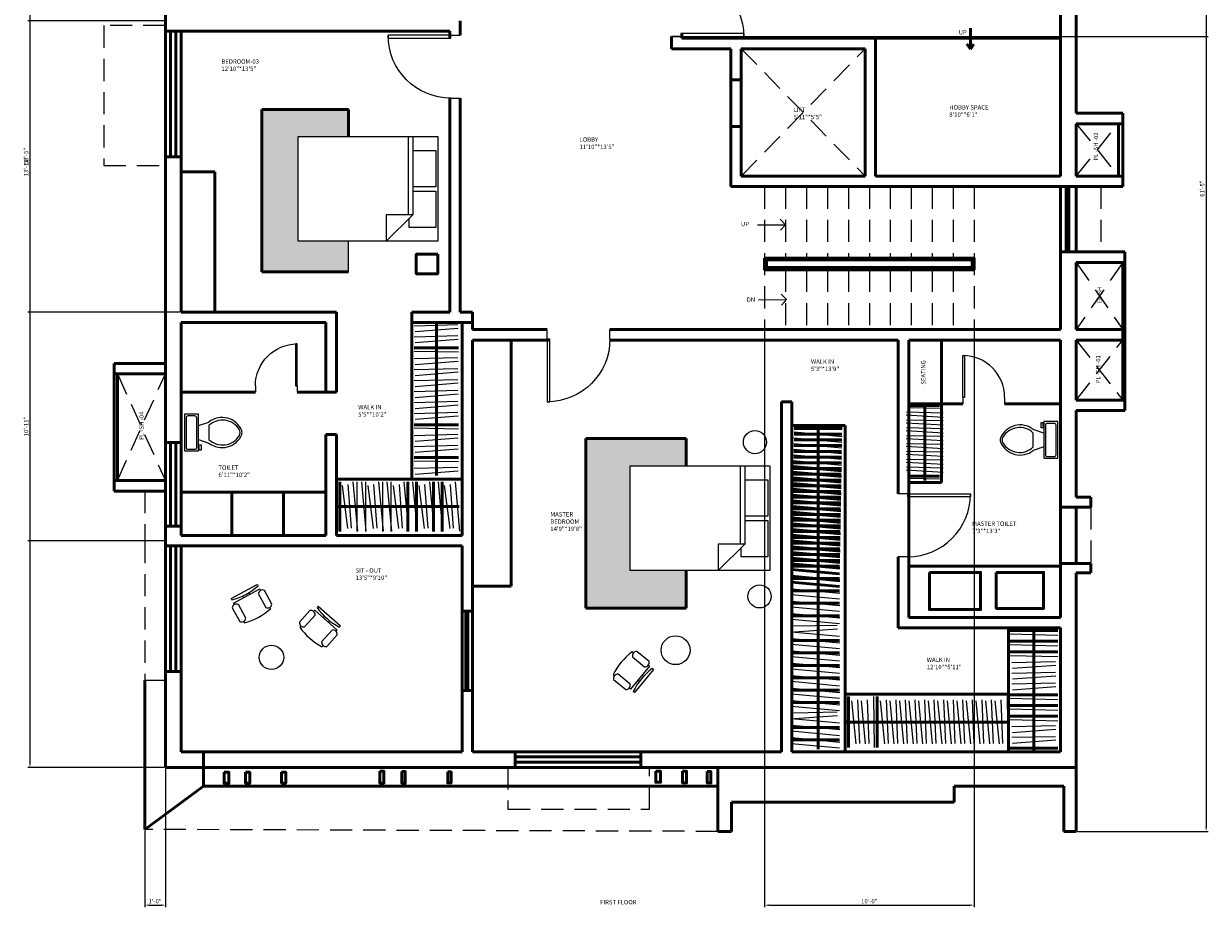
# Model space of a CAD drawing. Units: inches. Extents: x 5312 to 23584, y 2846 to 7447.
# Tile 5 of 12: x 9893 to 10572, y 3045 to 3551. Entities that reach past the tile are written whole.
import ezdxf

# ---------------------------------------------------------------- set-up
doc = ezdxf.new("R2010")
doc.units = ezdxf.units.IN
doc.linetypes.add('DASHED', pattern=[19.05, 12.7, -6.35])
for name, color, linetype, lineweight in [('A-ANNO-DIMS', 2, 'Continuous', 18), ('A-ANNO-TEXT', 3, 'Continuous', 18), ('A-AREA-IDEN', 7, 'Continuous', 18), ('A-DOOR', 4, 'Continuous', 25), ('A-FLOR-FIXT', 9, 'Continuous', 18), ('A-FLOR-OVHD', 8, 'DASHED', 18), ('A-FLOR-PATT', 252, 'Continuous', 13), ('A-FLOR-STRS', 3, 'Continuous', 18), ('A-FURN', 8, 'Continuous', 18), ('A-WALL', 7, 'Continuous', 50)]:
    doc.layers.add(name, color=color, linetype=linetype, lineweight=lineweight)
doc.styles.get("Standard").update_dxf_attribs({"font": 'arial.ttf'})
doc.dimstyles.new('ISO-25', dxfattribs={"dimtxt": 2.5, "dimasz": 2.5, "dimexe": 1.25, "dimexo": 0.625, "dimtad": 1, "dimlunit": 3, "dimtxsty": 'Standard', "dimcen": 2.5, "dimadec": 0, "dimazin": 0, "dimtfac": 1, "dimtmove": 0, "dimatfit": 3, "dimfxl": 1, "dimarcsym": 0})

# ---------------------------------------------------------------- blocks, each defined once
blk = doc.blocks.new('*U2')
for p, q in [((0, 0), (0, -6)), ((40, 0), (40, -6))]:
    blk.add_line(p, q)
blk.add_lwpolyline([(0, 0), (0, 40), (1.75, 40), (1.75, 0)], close=True)
blk.add_arc((0, 0), 40, 0, 90)
blk = doc.blocks.new('Toilet - top')
for p, q in [((9.5, -6), (9.5, -2)), ((-10, -8.5), (-8, -8.5)), ((-10, -9.5), (-10, -8.5)), ((-7, -9.5), (-10, -9.5)), ((-8, -8.5), (-8, -8)), ((-7, -8), (-7, -9.5)), ((-4, -8), (-6, -14)), ((4, -8), (6, -14)), ((4, -14), (-4, -14))]:
    blk.add_line(p, q)
blk.add_lwpolyline([(10.5, -8), (10.5, 0), (-10.5, 0), (-10.5, -8)], close=True)
for points in [[(-9.5, -2), (-9.5, -6)], [(8.5, -1), (-8.5, -1)], [(-8.5, -7), (8.5, -7)]]:
    blk.add_lwpolyline(points)
for centre, radius, start, end in [((-8.62, -1.88), 0.884, 81.8699, 188.1301), ((-8.62, -6.12), 0.884, 171.8699, 278.1301), ((8.62, -1.88), 0.884, 351.8699, 98.1301), ((8.62, -6.12), 0.884, 261.8699, 8.1301), ((3.52, -21.58), 12.17, 141.46911, 247.97143), ((4.2, -21.82), 11.33, 136.36773, 238.94682), ((-3.52, -21.58), 12.17, 292.02843, 38.53071), ((-4.2, -21.82), 11.33, 301.05301, 43.63209), ((0, -27.88), 4, 245.73182, 294.26817), ((0, -29), 4, 254.86053, 285.13947)]:
    blk.add_arc(centre, radius, start, end)
blk = doc.blocks.new('Bed - Queen')
for p, q in [((0, -80.00003), (0, 0)), ((0, 0), (59.99999, 0)), ((59.99999, 0), (59.99999, -80.00003)), ((7.99999, -1.2), (28.79998, -1.2)), ((7.99999, -14.4), (7.99999, -1.2)), ((28.79998, -1.2), (28.79998, -14.4)), ((31.19999, -1.2), (51.99999, -1.2)), ((31.19999, -14.4), (31.19999, -1.2)), ((51.99999, -1.2), (51.99999, -16.4)), ((0, -14.4), (44.8, -14.4)), ((44.8, -16.8), (0, -16.8)), ((59.99999, -29.6), (44.8, -14.4)), ((44.8, -14.4), (44.8, -29.6)), ((51.99999, -16.4), (46.79936, -16.4)), ((44.8, -29.6), (59.99999, -29.6)), ((59.99999, -80.00003), (0, -80.00003))]:
    blk.add_line(p, q)
blk = doc.blocks.new('Chair - Desk')
for p, q in [((-8.5, 0), (-8.5, -1)), ((-8.5, 0), (8.5, 0)), ((8.5, 0), (8.5, -1)), ((-10.5, -5), (-10.5, -14)), ((-8.5, -3), (-8.5, -4)), ((-8.5, -3), (8.5, -3)), ((-6.5, -14), (-6.5, -5)), ((-2, -3), (-2, -1.9355)), ((2, -1.9576), (2, -3)), ((6.5, -5), (6.5, -14)), ((8.5, -3), (8.5, -4)), ((10.5, -14), (10.5, -5)), ((-8.5, -15), (-8.5, -16)), ((8.5, -15), (8.5, -16))]:
    blk.add_line(p, q)
for centre, radius, start, end in [((-8.5, -6.5), 2.5, 36.8699, 143.1301), ((0, 34.625), 36.625, 256.5803, 283.4197), ((8.5, -6.5), 2.5, 36.8699, 143.1301), ((-8.5, -12.5), 2.5, 216.8699, 323.1301), ((0, 19.625), 36.625, 256.5803, 283.4197), ((8.5, -12.5), 2.5, 216.8699, 323.1301)]:
    blk.add_arc(centre, radius, start, end)
blk = doc.blocks.new('WARDROBE-HANGER')
for p, q in [((0, 3.4), (24.8, 3.4)), ((0, 1.32), (24.99, 0))]:
    blk.add_line(p, q)
blk = doc.blocks.new('WARDROBE-HANGER-B')
for p, q in [((0, 21.08), (0.79, 0)), ((2.48, 21.08), (2.48, 0))]:
    blk.add_line(p, q)
blk = doc.blocks.new('STAIR-ARROW')
for p, q in [((0, 3.17), (16.03, 3.17)), ((16.03, 3.17), (12.89, 6.38)), ((16.03, 3.17), (13.15, 0))]:
    blk.add_line(p, q)
blk = doc.blocks.new('*D72')
at = {"layer": 'A-ANNO-DIMS', "color": 0, "lineweight": -2, "transparency": 16777216}
for p, q in [((10497.49, 3825.38), (10572.19, 3825.38)), ((10570.94, 3822.88), (10570.94, 3090.84)), ((10497.14, 3088.34), (10572.19, 3088.34))]:
    blk.add_line(p, q, dxfattribs=at)
at = {"layer": 'A-ANNO-DIMS', "color": 0, "transparency": 16777216}
for points in [[(10570.52, 3822.88), (10571.35, 3822.88), (10570.94, 3825.38)], [(10570.52, 3090.84), (10571.35, 3090.84), (10570.94, 3088.34)]]:
    blk.add_solid(points, dxfattribs=at)
at = {"layer": 'DEFPOINTS', "color": 0, "transparency": 16777216}
for p in [(10496.86, 3825.38), (10496.51, 3088.34), (10570.94, 3088.34)]:
    blk.add_point(p, dxfattribs=at)
at = {"layer": 'A-ANNO-DIMS', "color": 0, "transparency": 16777216, "insert": (10569.03, 3456.86), "char_height": 2.5, "attachment_point": 5, "rotation": 90}
blk.add_mtext('61\'-5"', dxfattribs=at)
blk = doc.blocks.new('*D73')
at = {"layer": 'A-ANNO-DIMS', "color": 0, "lineweight": -2, "transparency": 16777216}
for p, q in [((9973.89, 3826.04), (9895.66, 3826.04)), ((9896.91, 3823.54), (9896.91, 3127.54)), ((9973.89, 3125.04), (9895.66, 3125.04))]:
    blk.add_line(p, q, dxfattribs=at)
at = {"layer": 'A-ANNO-DIMS', "color": 0, "transparency": 16777216}
for points in [[(9896.49, 3823.54), (9897.32, 3823.54), (9896.91, 3826.04)], [(9896.49, 3127.54), (9897.32, 3127.54), (9896.91, 3125.04)]]:
    blk.add_solid(points, dxfattribs=at)
at = {"layer": 'DEFPOINTS', "color": 0, "transparency": 16777216}
for p in [(9974.51, 3826.04), (9896.91, 3125.04), (9974.51, 3125.04)]:
    blk.add_point(p, dxfattribs=at)
at = {"layer": 'A-ANNO-DIMS', "color": 0, "transparency": 16777216, "insert": (9895.01, 3475.54), "char_height": 2.5, "attachment_point": 5, "rotation": 90}
blk.add_mtext('58\'-5"', dxfattribs=at)
blk = doc.blocks.new('*D77')
at = {"layer": 'A-ANNO-DIMS', "color": 0, "lineweight": -2, "transparency": 16777216}
for p, q in [((9973.89, 3553.04), (9895.66, 3553.04)), ((9896.91, 3550.54), (9896.91, 3388.54)), ((9982.89, 3386.04), (9895.66, 3386.04))]:
    blk.add_line(p, q, dxfattribs=at)
at = {"layer": 'A-ANNO-DIMS', "color": 0, "transparency": 16777216}
for points in [[(9896.49, 3550.54), (9897.32, 3550.54), (9896.91, 3553.04)], [(9896.49, 3388.54), (9897.32, 3388.54), (9896.91, 3386.04)]]:
    blk.add_solid(points, dxfattribs=at)
at = {"layer": 'DEFPOINTS', "color": 0, "transparency": 16777216}
for p in [(9974.51, 3553.04), (9896.91, 3386.04), (9983.51, 3386.04)]:
    blk.add_point(p, dxfattribs=at)
at = {"layer": 'A-ANNO-DIMS', "color": 0, "transparency": 16777216, "insert": (9895.01, 3469.54), "char_height": 2.5, "attachment_point": 5, "rotation": 90}
blk.add_mtext('13\'-11"', dxfattribs=at)
blk = doc.blocks.new('*D78')
at = {"layer": 'A-ANNO-DIMS', "color": 0, "lineweight": -2, "transparency": 16777216}
for p, q in [((9982.89, 3386.04), (9895.66, 3386.04)), ((9896.91, 3383.54), (9896.91, 3257.42)), ((9973.89, 3254.92), (9895.66, 3254.92))]:
    blk.add_line(p, q, dxfattribs=at)
at = {"layer": 'A-ANNO-DIMS', "color": 0, "transparency": 16777216}
for points in [[(9896.49, 3383.54), (9897.32, 3383.54), (9896.91, 3386.04)], [(9896.49, 3257.42), (9897.32, 3257.42), (9896.91, 3254.92)]]:
    blk.add_solid(points, dxfattribs=at)
at = {"layer": 'DEFPOINTS', "color": 0, "transparency": 16777216}
for p in [(9983.51, 3386.04), (9896.91, 3254.92), (9974.51, 3254.92)]:
    blk.add_point(p, dxfattribs=at)
at = {"layer": 'A-ANNO-DIMS', "color": 0, "transparency": 16777216, "insert": (9895.01, 3320.48), "char_height": 2.5, "attachment_point": 5, "rotation": 90}
blk.add_mtext('10\'-11"', dxfattribs=at)
blk = doc.blocks.new('*D79')
at = {"layer": 'A-ANNO-DIMS', "color": 0, "lineweight": -2, "transparency": 16777216}
for p, q in [((9974.51, 3124.42), (9974.51, 3044.84)), ((9962.67, 3088.84), (9962.67, 3044.84)), ((9965.17, 3046.09), (9972.01, 3046.09))]:
    blk.add_line(p, q, dxfattribs=at)
at = {"layer": 'A-ANNO-DIMS', "color": 0, "transparency": 16777216}
for points in [[(9965.17, 3046.51), (9965.17, 3045.67), (9962.67, 3046.09)], [(9972.01, 3046.51), (9972.01, 3045.67), (9974.51, 3046.09)]]:
    blk.add_solid(points, dxfattribs=at)
at = {"layer": 'DEFPOINTS', "color": 0, "transparency": 16777216}
for p in [(9974.51, 3125.04), (9962.67, 3089.46), (9974.51, 3046.09)]:
    blk.add_point(p, dxfattribs=at)
at = {"layer": 'A-ANNO-DIMS', "color": 0, "transparency": 16777216, "insert": (9968.59, 3047.99), "char_height": 2.5, "attachment_point": 5}
blk.add_mtext('1\'-0"', dxfattribs=at)
blk = doc.blocks.new('*D81')
at = {"layer": 'A-ANNO-DIMS', "color": 0, "lineweight": -2, "transparency": 16777216}
for p, q in [((10317.93, 3375.42), (10317.93, 3044.84)), ((10437.93, 3375.42), (10437.93, 3044.84)), ((10320.43, 3046.09), (10435.43, 3046.09))]:
    blk.add_line(p, q, dxfattribs=at)
at = {"layer": 'A-ANNO-DIMS', "color": 0, "transparency": 16777216}
for points in [[(10320.43, 3046.51), (10320.43, 3045.67), (10317.93, 3046.09)], [(10435.43, 3046.51), (10435.43, 3045.67), (10437.93, 3046.09)]]:
    blk.add_solid(points, dxfattribs=at)
at = {"layer": 'DEFPOINTS', "color": 0, "transparency": 16777216}
for p in [(10317.93, 3376.04), (10437.93, 3376.04), (10437.93, 3046.09)]:
    blk.add_point(p, dxfattribs=at)
at = {"layer": 'A-ANNO-DIMS', "color": 0, "transparency": 16777216, "insert": (10377.93, 3047.99), "char_height": 2.5, "attachment_point": 5}
blk.add_mtext('10\'-0"', dxfattribs=at)
blk = doc.blocks.new('*D82')
at = {"layer": 'A-ANNO-DIMS', "color": 0, "lineweight": -2, "transparency": 16777216}
for p, q in [((10265.14, 3580.12), (10572.19, 3580.12)), ((10570.94, 3577.62), (10570.94, 3546.62)), ((10265.14, 3544.12), (10572.19, 3544.12))]:
    blk.add_line(p, q, dxfattribs=at)
at = {"layer": 'A-ANNO-DIMS', "color": 0, "transparency": 16777216}
for points in [[(10570.52, 3577.62), (10571.35, 3577.62), (10570.94, 3580.12)], [(10570.52, 3546.62), (10571.35, 3546.62), (10570.94, 3544.12)]]:
    blk.add_solid(points, dxfattribs=at)
at = {"layer": 'DEFPOINTS', "color": 0, "transparency": 16777216}
for p in [(10264.51, 3580.12), (10264.51, 3544.12), (10570.94, 3544.12)]:
    blk.add_point(p, dxfattribs=at)
at = {"layer": 'A-ANNO-DIMS', "color": 0, "transparency": 16777216, "insert": (10569.03, 3562.12), "char_height": 2.5, "attachment_point": 5, "rotation": 90}
blk.add_mtext('3\'-0"', dxfattribs=at)

msp = doc.modelspace()

# ---------------------------------------------------------------- hatches: boundary and pattern name
at = {"layer": 'A-FLOR-PATT'}
h = msp.add_hatch(dxfattribs=at)
h.set_pattern_fill('STARS', color=256)
h.set_pattern_definition([(0, (143.128, -197.685), (0, 5.4992613), [3.175, -3.175]), (60, (143.128, -197.685), (-4.7625, 2.7496307), [3.175, -3.175]), (120, (144.716, -194.935), (-4.7625, -2.7496307), [3.175, -3.175])])
h.paths.add_polyline_path([(10050.622, 3486.666), (10079.433, 3486.666), (10079.433, 3502.163), (10029.764, 3502.163), (10029.764, 3409.236), (10079.433, 3409.236), (10079.433, 3426.666), (10050.622, 3426.666)])
h.paths.add_polyline_path([(10240.933, 3297.856), (10272.957, 3297.856), (10272.957, 3313.673), (10215.389, 3313.673), (10215.389, 3216.331), (10272.957, 3216.331), (10272.957, 3237.856), (10240.933, 3237.856)])

# ---------------------------------------------------------------- linework, layer by layer
at = {"layer": 'A-FLOR-OVHD'}
for p, q in [((9974.514, 3550.302), (9939.158, 3550.302)), ((9939.158, 3550.302), (9939.158, 3470.121)), ((10304.514, 3537.044), (10375.514, 3464.044)), ((10304.514, 3464.044), (10375.514, 3537.044)), ((10496.514, 3494.066), (10520.654, 3464.044)), ((10496.514, 3464.044), (10520.654, 3494.066)), ((9939.158, 3470.121), (9974.514, 3470.121)), ((10317.934, 3458.044), (10317.934, 3376.044)), ((10329.934, 3458.044), (10329.934, 3417.044)), ((10341.934, 3458.044), (10341.934, 3417.044)), ((10353.934, 3458.044), (10353.934, 3417.044)), ((10365.934, 3458.044), (10365.934, 3417.044)), ((10377.934, 3458.044), (10377.934, 3417.044)), ((10389.934, 3458.044), (10389.934, 3417.044)), ((10401.934, 3458.044), (10401.934, 3417.044)), ((10413.934, 3458.044), (10413.934, 3417.044)), ((10425.934, 3458.044), (10425.934, 3417.044)), ((10437.934, 3458.044), (10437.934, 3376.044)), ((10510.672, 3458.044), (10510.672, 3420.542)), ((10329.934, 3410.329), (10329.934, 3376.044)), ((10341.934, 3410.329), (10341.934, 3376.044)), ((10353.934, 3410.329), (10353.934, 3376.044)), ((10365.934, 3410.329), (10365.934, 3376.044)), ((10377.934, 3410.329), (10377.934, 3376.044)), ((10389.934, 3410.329), (10389.934, 3376.044)), ((10401.934, 3410.329), (10401.934, 3376.044)), ((10413.934, 3410.329), (10413.934, 3376.044)), ((10425.934, 3410.329), (10425.934, 3376.044)), ((10496.514, 3414.542), (10523.189, 3376.044)), ((10523.189, 3414.542), (10496.514, 3376.044)), ((10496.514, 3370.044), (10523.189, 3335.57)), ((10496.514, 3335.57), (10523.189, 3370.036)), ((9946.998, 3350.695), (9974.514, 3289.508)), ((9946.998, 3289.508), (9974.514, 3350.695)), ((9962.667, 3283.508), (9962.667, 3254.921)), ((10504.83, 3274.199), (10504.83, 3241.979)), ((9974.514, 3254.921), (9962.667, 3254.921)), ((9962.667, 3254.921), (9962.667, 3175.011)), ((9962.667, 3175.011), (9974.514, 3175.011)), ((9962.667, 3175.011), (9962.667, 3175.011)), ((10170.825, 3125.044), (10170.825, 3101.018)), ((10252.016, 3101.018), (10252.016, 3125.044)), ((10170.825, 3101.018), (10252.016, 3101.018)), ((10291.107, 3088.341), (9962.667, 3089.464))]:
    msp.add_line(p, q, dxfattribs=at)
at = {"layer": 'A-FURN'}
for p, q in [((10079.433, 3409.236), (10079.433, 3426.666)), ((10117.106, 3363.712), (10142.474, 3363.209)), ((10401.356, 3331.474), (10418.069, 3331.007)), ((10117.106, 3319.708), (10142.474, 3319.205)), ((10334.705, 3314.069), (10362.225, 3311.557)), ((10334.762, 3317.357), (10362.282, 3314.845)), ((10334.591, 3307.492), (10362.112, 3304.98)), ((10334.648, 3310.78), (10362.169, 3308.268)), ((10117.106, 3300.848), (10142.474, 3300.346)), ((10334.478, 3300.916), (10361.998, 3298.404)), ((10334.534, 3304.204), (10362.055, 3301.692)), ((10081.957, 3288.687), (10084.58, 3260.422)), ((10084.26, 3288.687), (10084.26, 3260.377)), ((10086.836, 3288.687), (10089.46, 3260.422)), ((10089.14, 3288.687), (10089.14, 3260.377)), ((10096.596, 3288.687), (10099.219, 3260.422)), ((10098.899, 3288.687), (10098.899, 3260.377)), ((10101.475, 3288.687), (10104.099, 3260.422)), ((10103.779, 3288.687), (10103.779, 3260.377)), ((10111.235, 3288.687), (10113.858, 3260.422)), ((10116.114, 3288.687), (10118.738, 3260.422)), ((10125.874, 3288.687), (10128.497, 3260.422)), ((10130.754, 3288.687), (10133.377, 3260.422)), ((10140.513, 3288.687), (10143.136, 3260.422)), ((10401.356, 3290.93), (10418.069, 3290.462)), ((10333.455, 3227.496), (10360.976, 3224.984)), ((10333.398, 3224.208), (10360.919, 3221.696)), ((10333.455, 3220.38), (10360.976, 3217.868)), ((10333.398, 3217.092), (10360.919, 3214.58)), ((10333.455, 3213.264), (10360.976, 3210.752)), ((10333.398, 3209.976), (10360.919, 3207.464)), ((10333.398, 3202.86), (10360.919, 3200.348)), ((10333.455, 3199.033), (10360.976, 3196.521)), ((10458.651, 3201.569), (10485.908, 3200.861)), ((10333.398, 3195.745), (10360.919, 3193.233)), ((10333.455, 3191.917), (10360.976, 3189.405)), ((10458.651, 3195.433), (10485.908, 3194.726)), ((10333.398, 3188.629), (10360.919, 3186.117)), ((10333.455, 3184.801), (10360.976, 3182.289)), ((10458.651, 3189.298), (10485.908, 3188.59)), ((10333.398, 3181.513), (10360.919, 3179.001)), ((10333.455, 3177.685), (10360.976, 3175.173)), ((10333.398, 3174.397), (10360.919, 3171.885)), ((10333.455, 3170.57), (10360.976, 3168.058)), ((10333.398, 3167.281), (10360.919, 3164.769)), ((10380.311, 3165.638), (10380.704, 3136.514)), ((10456.955, 3165.638), (10457.348, 3136.514)), ((10458.651, 3164.755), (10485.908, 3164.047)), ((10333.398, 3160.166), (10360.919, 3157.654)), ((10333.455, 3163.454), (10360.976, 3160.942)), ((10458.651, 3158.619), (10485.908, 3157.911)), ((10333.398, 3153.05), (10360.919, 3150.538)), ((10458.651, 3152.483), (10485.908, 3151.776)), ((10333.398, 3145.934), (10360.919, 3143.422)), ((10333.455, 3149.222), (10360.976, 3146.71)), ((10333.398, 3138.818), (10360.919, 3136.306)), ((10333.455, 3142.106), (10360.976, 3139.594)), ((10458.651, 3134.076), (10485.908, 3133.369))]:
    msp.add_line(p, q, dxfattribs=at)
for centre, radius in [((10312.362, 3311.539), 6.627), ((10315.013, 3223.081), 6.627), ((10266.896, 3192.222), 8.269), ((10035.309, 3188.14), 7.003)]:
    msp.add_circle(centre, radius, dxfattribs=at)
at = {"layer": 'A-WALL'}
for p, q in [((9974.514, 3826.044), (9974.514, 3125.044)), ((10487.514, 3722.044), (10487.514, 3464.044)), ((10496.514, 3715.012), (10496.514, 3500.066)), ((10143.514, 3553.044), (10143.514, 3544.747)), ((9974.514, 3475.052), (9974.514, 3547.052)), ((9974.514, 3547.052), (9983.514, 3547.052)), ((10137.514, 3547.044), (9974.514, 3547.044)), ((9977.514, 3475.052), (9977.514, 3547.052)), ((9980.514, 3547.052), (9980.514, 3475.052)), ((9983.514, 3547.052), (9983.514, 3475.052)), ((9983.514, 3547.052), (9983.514, 3386.044)), ((10137.514, 3547.044), (10137.514, 3543.172)), ((10264.514, 3544.118), (10264.514, 3537.044)), ((10270.514, 3545.693), (10270.514, 3543.044)), ((10435.977, 3548.871), (10435.977, 3536.826)), ((10264.514, 3537.044), (10298.514, 3537.044)), ((10270.514, 3543.044), (10487.514, 3543.044)), ((10298.514, 3537.044), (10298.514, 3458.044)), ((10304.514, 3537.044), (10304.514, 3464.044)), ((10304.514, 3537.044), (10375.514, 3537.044)), ((10375.514, 3537.044), (10375.514, 3464.044)), ((10381.514, 3543.044), (10381.514, 3464.044)), ((10435.977, 3536.826), (10433.765, 3539.791)), ((10435.977, 3536.826), (10437.721, 3539.744)), ((10298.514, 3519.288), (10304.514, 3519.288)), ((10137.514, 3508.752), (10137.514, 3386.044)), ((10143.514, 3508.747), (10143.514, 3386.044)), ((10079.433, 3502.163), (10029.764, 3502.163)), ((10029.764, 3502.163), (10029.764, 3409.236)), ((10079.433, 3486.666), (10079.433, 3502.163)), ((10520.654, 3500.066), (10496.514, 3500.066)), ((10520.654, 3500.066), (10523.25, 3500.066)), ((10523.25, 3500.066), (10523.25, 3458.044)), ((10298.514, 3492.519), (10304.514, 3492.519)), ((10523.25, 3494.066), (10496.514, 3494.066)), ((10496.514, 3494.066), (10496.514, 3464.044)), ((10520.654, 3464.044), (10520.654, 3494.066)), ((10520.654, 3494.066), (10520.654, 3494.066)), ((9983.514, 3475.052), (9974.514, 3475.052)), ((9983.514, 3466.548), (10002.874, 3466.548)), ((10002.874, 3466.548), (10002.874, 3386.044)), ((10304.514, 3464.044), (10375.514, 3464.044)), ((10381.514, 3464.044), (10487.514, 3464.044)), ((10523.25, 3464.044), (10496.514, 3464.044)), ((10298.514, 3458.044), (10496.514, 3458.044)), ((10487.514, 3458.044), (10487.514, 3376.044)), ((10490.706, 3458.044), (10490.706, 3420.542)), ((10492.205, 3458.044), (10492.205, 3420.542)), ((10496.514, 3458.044), (10520.654, 3458.044)), ((10496.514, 3458.044), (10496.514, 3420.542)), ((10523.25, 3458.044), (10520.654, 3458.044)), ((10496.405, 3420.542), (10487.514, 3420.542)), ((10496.405, 3420.542), (10523.189, 3420.542)), ((10523.189, 3420.542), (10524.356, 3420.542)), ((10524.356, 3420.542), (10524.356, 3329.57)), ((10029.764, 3409.236), (10079.433, 3409.236)), ((10496.514, 3414.542), (10524.356, 3414.542)), ((10496.514, 3414.542), (10496.514, 3376.044)), ((10523.189, 3414.542), (10523.189, 3335.57)), ((10072.514, 3386.044), (9983.514, 3386.044)), ((10072.514, 3386.044), (10072.514, 3340.211)), ((10137.514, 3386.044), (10115.78, 3386.044)), ((10115.78, 3386.044), (10115.78, 3290.337)), ((10150.514, 3386.044), (10143.514, 3386.044)), ((10150.514, 3386.044), (10150.514, 3376.044)), ((9983.514, 3380.044), (9983.514, 3258.044)), ((10066.514, 3380.044), (9983.514, 3380.044)), ((10066.514, 3380.044), (10066.514, 3340.211)), ((10150.514, 3380.044), (10115.78, 3380.044)), ((10129.79, 3379.221), (10129.79, 3292.433)), ((10144.514, 3380.044), (10144.514, 3258.044)), ((10150.514, 3376.044), (10193.289, 3376.044)), ((10229.289, 3376.044), (10487.514, 3376.044)), ((10496.514, 3376.044), (10523.189, 3376.044)), ((10150.514, 3370.044), (10194.864, 3370.044)), ((10150.514, 3370.044), (10150.514, 3134.044)), ((10172.634, 3370.044), (10172.634, 3228.941)), ((10229.284, 3370.044), (10333.514, 3370.044)), ((10333.514, 3370.044), (10394.514, 3370.044)), ((10394.514, 3370.044), (10394.514, 3281.83)), ((10400.514, 3370.044), (10400.514, 3211.044)), ((10400.514, 3370.044), (10487.514, 3370.044)), ((10419.245, 3370.044), (10419.245, 3370.044)), ((10419.245, 3370.044), (10419.245, 3288.315)), ((10487.514, 3370.044), (10487.514, 3211.044)), ((10496.514, 3370.044), (10523.189, 3370.044)), ((10496.514, 3370.044), (10496.514, 3335.57)), ((10117.106, 3365.501), (10142.474, 3365.501)), ((9974.514, 3356.695), (9945.182, 3356.695)), ((9945.182, 3356.695), (9945.182, 3283.508)), ((9974.514, 3350.695), (9945.182, 3350.695)), ((9946.998, 3350.695), (9946.998, 3289.508)), ((9983.514, 3340.211), (9986.306, 3340.211)), ((9986.306, 3340.211), (10026.091, 3340.211)), ((10050.091, 3340.211), (10066.514, 3340.211)), ((10066.514, 3340.211), (10066.514, 3340.211)), ((10066.514, 3340.211), (10072.514, 3340.211)), ((10327.514, 3334.602), (10327.514, 3134.044)), ((10327.514, 3334.602), (10333.514, 3334.602)), ((10333.514, 3334.602), (10333.514, 3134.044)), ((10419.245, 3333.565), (10400.514, 3333.565)), ((10431.478, 3333.565), (10419.245, 3333.565)), ((10455.478, 3333.565), (10487.514, 3333.565)), ((10496.514, 3335.57), (10524.356, 3335.57)), ((10401.174, 3332.541), (10401.242, 3332.541)), ((10401.174, 3331.501), (10401.356, 3331.474)), ((10401.242, 3332.541), (10418.069, 3332.541)), ((10409.655, 3333.069), (10409.655, 3289.584)), ((10496.514, 3329.57), (10523.189, 3329.57)), ((10496.514, 3329.57), (10496.514, 3279.966)), ((10524.356, 3329.57), (10523.189, 3329.57)), ((10117.106, 3321.496), (10142.474, 3321.496)), ((10333.514, 3321.111), (10364.095, 3321.111)), ((10348.579, 3320.476), (10348.579, 3135.553)), ((10364.095, 3321.111), (10364.095, 3134.044)), ((10066.514, 3315.899), (10072.514, 3315.899)), ((10066.514, 3315.899), (10066.514, 3258.044)), ((10072.514, 3315.899), (10072.514, 3258.044)), ((10272.957, 3313.673), (10215.389, 3313.673)), ((10215.389, 3313.673), (10215.389, 3216.331)), ((10272.957, 3297.856), (10272.957, 3313.673)), ((10334.762, 3319.389), (10334.875, 3319.389)), ((10334.818, 3316.101), (10362.225, 3316.101)), ((10334.875, 3319.389), (10362.282, 3319.389)), ((9974.514, 3263.339), (9974.514, 3311.339)), ((9974.514, 3311.339), (9983.514, 3311.339)), ((9977.514, 3263.339), (9977.514, 3311.339)), ((9980.514, 3311.339), (9980.514, 3263.339)), ((9983.514, 3311.339), (9983.514, 3263.339)), ((10334.648, 3306.236), (10362.055, 3306.236)), ((10334.705, 3309.524), (10362.112, 3309.524)), ((10334.762, 3312.813), (10362.169, 3312.813)), ((10117.106, 3302.637), (10142.474, 3302.637)), ((10334.534, 3299.66), (10361.941, 3299.66)), ((10334.591, 3302.948), (10361.998, 3302.948)), ((10334.364, 3294.339), (10361.885, 3291.827)), ((10334.421, 3297.627), (10361.941, 3295.115)), ((10334.421, 3293.083), (10361.828, 3293.083)), ((10334.478, 3296.371), (10361.885, 3296.371)), ((9945.182, 3289.508), (9974.514, 3289.508)), ((10072.514, 3290.337), (10144.514, 3290.337)), ((10074.5, 3288.687), (10074.5, 3260.377)), ((10113.538, 3288.687), (10113.538, 3260.377)), ((10118.418, 3288.687), (10118.418, 3260.377)), ((10128.177, 3288.687), (10128.177, 3260.377)), ((10133.057, 3288.687), (10133.057, 3260.377)), ((10334.25, 3287.763), (10361.771, 3285.251)), ((10334.307, 3291.051), (10361.828, 3288.539)), ((10334.307, 3286.507), (10361.714, 3286.507)), ((10334.364, 3289.795), (10361.771, 3289.795)), ((10419.245, 3288.315), (10400.514, 3288.315)), ((10401.242, 3291.997), (10418.069, 3291.997)), ((9945.182, 3283.508), (9974.514, 3283.508)), ((9983.514, 3282.76), (10066.514, 3282.76)), ((10334.137, 3281.186), (10361.657, 3278.674)), ((10334.194, 3284.475), (10361.714, 3281.962)), ((10334.194, 3279.93), (10361.601, 3279.93)), ((10334.25, 3283.218), (10361.657, 3283.218)), ((10504.83, 3279.966), (10496.514, 3279.966)), ((10504.83, 3274.199), (10504.83, 3279.966)), ((10073.465, 3274.532), (10142.928, 3274.532)), ((10334.023, 3274.61), (10361.544, 3272.098)), ((10334.08, 3277.898), (10361.601, 3275.386)), ((10334.08, 3273.354), (10361.487, 3273.354)), ((10334.137, 3276.642), (10361.544, 3276.642)), ((10487.514, 3274.199), (10504.83, 3274.199)), ((10496.514, 3274.199), (10496.514, 3241.979)), ((10333.91, 3268.033), (10361.43, 3265.521)), ((10333.966, 3271.322), (10361.487, 3268.81)), ((10333.966, 3266.777), (10361.373, 3266.777)), ((10334.023, 3270.066), (10361.43, 3270.066)), ((9983.514, 3263.339), (9974.514, 3263.339)), ((10333.796, 3261.457), (10361.317, 3258.945)), ((10333.853, 3264.745), (10361.373, 3262.233)), ((10333.853, 3260.201), (10361.26, 3260.201)), ((10333.91, 3263.489), (10361.317, 3263.489)), ((10144.514, 3252.044), (9974.514, 3252.044)), ((9974.514, 3180.044), (9974.514, 3252.044)), ((9974.514, 3252.044), (9983.514, 3252.044)), ((9977.514, 3180.044), (9977.514, 3252.044)), ((9980.514, 3252.044), (9980.514, 3180.044)), ((10066.514, 3258.044), (9983.514, 3258.044)), ((9983.514, 3252.044), (9983.514, 3180.044)), ((9983.514, 3252.044), (9983.514, 3134.044)), ((10144.514, 3258.044), (10072.514, 3258.044)), ((10144.514, 3252.044), (10144.514, 3134.044)), ((10333.682, 3254.88), (10361.203, 3252.368)), ((10333.739, 3258.169), (10361.26, 3255.657)), ((10333.739, 3253.624), (10361.146, 3253.624)), ((10333.796, 3256.913), (10361.203, 3256.913)), ((10333.569, 3248.304), (10361.089, 3245.792)), ((10333.626, 3251.592), (10361.146, 3249.08)), ((10333.626, 3247.048), (10361.033, 3247.048)), ((10333.682, 3250.336), (10361.089, 3250.336)), ((10394.514, 3245.83), (10394.514, 3205.044)), ((10333.398, 3238.439), (10360.919, 3235.927)), ((10333.455, 3241.728), (10360.976, 3239.216)), ((10333.512, 3245.016), (10361.033, 3242.504)), ((10333.512, 3240.472), (10360.919, 3240.472)), ((10333.569, 3243.76), (10360.976, 3243.76)), ((10400.514, 3240.467), (10487.514, 3240.467)), ((10504.83, 3241.979), (10487.514, 3241.979)), ((10504.83, 3236.599), (10504.83, 3241.979)), ((10272.957, 3216.331), (10272.957, 3237.856)), ((10333.455, 3234.612), (10360.976, 3232.1)), ((10333.512, 3233.356), (10360.919, 3233.356)), ((10496.514, 3236.599), (10504.83, 3236.599)), ((10496.514, 3236.599), (10496.514, 3125.044)), ((10172.634, 3228.941), (10150.514, 3228.941)), ((10333.398, 3231.324), (10360.919, 3228.811)), ((10333.512, 3226.24), (10360.919, 3226.24)), ((10333.512, 3219.124), (10360.919, 3219.124)), ((10144.514, 3214.563), (10150.514, 3214.563)), ((10146.718, 3214.563), (10146.718, 3169.11)), ((10147.837, 3214.548), (10147.837, 3169.11)), ((10215.389, 3216.331), (10272.957, 3216.331)), ((10333.512, 3212.008), (10360.919, 3212.008)), ((10394.514, 3205.044), (10487.514, 3205.044)), ((10400.514, 3211.044), (10487.514, 3211.044)), ((10457.622, 3205.044), (10457.622, 3134.044)), ((10472.279, 3204.426), (10472.279, 3133.9)), ((10487.514, 3205.044), (10487.514, 3134.044)), ((10333.512, 3197.777), (10360.919, 3197.777)), ((10458.651, 3203.554), (10485.908, 3203.554)), ((10458.651, 3197.418), (10485.908, 3197.418)), ((10458.651, 3191.282), (10485.908, 3191.282)), ((10333.512, 3190.661), (10360.919, 3190.661)), ((9983.514, 3180.044), (9974.514, 3180.044)), ((10333.512, 3183.545), (10360.919, 3183.545)), ((9962.667, 3175.011), (9962.667, 3101.018)), ((10333.512, 3176.429), (10360.919, 3176.429)), ((10144.514, 3169.11), (10150.514, 3169.11)), ((10333.512, 3169.314), (10360.919, 3169.314)), ((10364.095, 3167.037), (10457.622, 3167.037)), ((10365.983, 3165.638), (10365.983, 3136.442)), ((10382.407, 3165.638), (10382.407, 3136.442)), ((10458.651, 3166.74), (10485.908, 3166.74)), ((10333.512, 3162.198), (10360.919, 3162.198)), ((10458.651, 3160.604), (10485.908, 3160.604)), ((10364.911, 3151.04), (10457.375, 3151.04)), ((10458.651, 3154.468), (10485.908, 3154.468)), ((10333.512, 3147.966), (10360.919, 3147.966)), ((10333.512, 3140.85), (10360.919, 3140.85)), ((10144.514, 3134.044), (9983.514, 3134.044)), ((9996.35, 3114.343), (9996.35, 3134.044)), ((10263.514, 3134.044), (10150.514, 3134.044)), ((10174.961, 3134.044), (10246.961, 3134.044)), ((10174.961, 3125.044), (10174.961, 3134.044)), ((10174.961, 3131.044), (10246.961, 3131.044)), ((10246.961, 3134.044), (10246.961, 3125.044)), ((10263.514, 3134.044), (10327.514, 3134.044)), ((10333.514, 3134.044), (10487.514, 3134.044)), ((10458.651, 3136.061), (10485.908, 3136.061)), ((10263.514, 3125.044), (9974.514, 3125.044)), ((10246.961, 3128.044), (10174.961, 3128.044)), ((10246.961, 3125.044), (10174.961, 3125.044)), ((10263.514, 3125.044), (10496.514, 3125.044)), ((10291.107, 3125.044), (10291.107, 3088.341)), ((10496.514, 3088.341), (10496.514, 3125.044)), ((9962.667, 3089.464), (9996.35, 3114.343)), ((9996.35, 3114.343), (10291.107, 3114.343)), ((10426.462, 3105.121), (10426.462, 3114.221)), ((10426.462, 3114.221), (10489.433, 3114.221)), ((10489.433, 3114.221), (10489.433, 3088.341)), ((10299.02, 3088.341), (10299.02, 3105.121)), ((10299.02, 3105.121), (10426.462, 3105.121)), ((9962.667, 3101.018), (9962.667, 3089.464)), ((10291.107, 3088.341), (10299.02, 3088.341)), ((10489.433, 3088.341), (10496.514, 3088.341))]:
    msp.add_line(p, q, dxfattribs=at)
for points in [[(10130.622, 3419.224), (10118.266, 3419.224), (10118.266, 3408.09), (10130.622, 3408.09)], [(10317.934, 3417.044), (10437.934, 3417.044), (10437.934, 3410.329), (10317.934, 3410.329)], [(10319, 3415.959), (10436.845, 3415.959), (10436.845, 3411.728), (10319, 3411.728)], [(10012.497, 3282.76), (10042.152, 3282.76), (10042.152, 3258.044), (10012.497, 3258.044)], [(10412.348, 3236.789), (10441.663, 3236.789), (10441.663, 3215.486), (10412.348, 3215.486)], [(10450.701, 3236.789), (10477.796, 3236.789), (10477.796, 3216.235), (10450.701, 3216.235)], [(10097.324, 3122.875), (10099.744, 3122.875), (10099.744, 3116.023), (10097.324, 3116.023)], [(10255.519, 3122.882), (10258.295, 3122.882), (10258.295, 3116.517), (10255.519, 3116.517)], [(10008.147, 3122.298), (10010.955, 3122.298), (10010.955, 3115.945), (10008.147, 3115.945)], [(10020.462, 3122.298), (10022.897, 3122.298), (10022.897, 3115.996), (10020.462, 3115.996)], [(10041.062, 3122.233), (10043.514, 3122.233), (10043.514, 3116.03), (10041.062, 3116.03)], [(10110.081, 3122.658), (10111.937, 3122.658), (10111.937, 3115.916), (10110.081, 3115.916)], [(10136.343, 3122.488), (10138.195, 3122.488), (10138.195, 3116.196), (10136.343, 3116.196)], [(10270.88, 3122.825), (10273.202, 3122.825), (10273.202, 3116.205), (10270.88, 3116.205)], [(10285.008, 3122.69), (10287.123, 3122.69), (10287.123, 3116.157), (10285.008, 3116.157)]]:
    msp.add_lwpolyline(points, close=True, dxfattribs=at)

# ---------------------------------------------------------------- block references
at = {"layer": 'A-DOOR', "yscale": 0.9, "zscale": 0.9}
for p, xscale, rotation in [((10269.914, 3544.118), -0.9, 270), ((10138.114, 3544.747), -0.9, 90), ((10193.289, 3370.644), -0.9, 180), ((10399.914, 3281.83), 0.9, 270)]:
    msp.add_blockref('*U2', p, dxfattribs=dict(at, xscale=xscale, rotation=rotation))
at = {"layer": 'A-DOOR', "yscale": 0.6, "zscale": 0.6}
for p, xscale in [((10050.091, 3343.811), -0.6), ((10431.478, 3337.165), 0.6)]:
    msp.add_blockref('*U2', p, dxfattribs=dict(at, xscale=xscale))
at = {"layer": 'A-FLOR-FIXT'}
for p, rotation in [((9985.444, 3317.01), 90), ((10485.91, 3312.758), 270)]:
    msp.add_blockref('Toilet - top', p, dxfattribs=dict(at, rotation=rotation))
at = {"layer": 'A-FLOR-STRS'}
msp.add_blockref('STAIR-ARROW', (10313.899, 3432.954), dxfattribs=at)
at = {"layer": 'A-FLOR-STRS', "rotation": 0.1925238956542199}
msp.add_blockref('STAIR-ARROW', (10314.508, 3390.015), dxfattribs=at)
at = {"layer": 'A-FURN'}
for name, p, rotation in [('Bed - Queen', (10130.622, 3486.666), 270), ('WARDROBE-HANGER', (10142.036, 3380.076), 184.5999666414178), ('WARDROBE-HANGER', (10142.036, 3373.79), 184.5999666414178), ('WARDROBE-HANGER', (10142.036, 3361.217), 184.5999666414178), ('WARDROBE-HANGER', (10142.036, 3354.931), 184.5999666414178), ('WARDROBE-HANGER', (10142.036, 3348.645), 184.5999666414178), ('WARDROBE-HANGER', (10142.036, 3342.358), 184.5999666414158), ('WARDROBE-HANGER', (10142.036, 3336.072), 184.5999666414178), ('WARDROBE-HANGER', (10142.036, 3329.786), 184.5999666414178), ('WARDROBE-HANGER-B', (10399.244, 3329.43), 266.6777617258486), ('WARDROBE-HANGER-B', (10399.244, 3324.925), 266.6777617258455), ('WARDROBE-HANGER-B', (10399.244, 3320.42), 266.6777617258455), ('WARDROBE-HANGER', (10142.036, 3317.213), 184.5999666414199), ('WARDROBE-HANGER-B', (10399.244, 3315.916), 266.6777617258486), ('WARDROBE-HANGER', (10142.036, 3310.927), 184.5999666414178), ('WARDROBE-HANGER-B', (10399.244, 3311.411), 266.6777617258486), ('WARDROBE-HANGER-B', (10399.244, 3306.906), 266.6777617258486), ('WARDROBE-HANGER-B', (10399.244, 3302.401), 266.6777617258486), ('WARDROBE-HANGER', (10142.036, 3298.354), 184.5999666414158), ('Bed - Queen', (10320.933, 3297.856), 270), ('WARDROBE-HANGER-B', (10399.244, 3297.896), 266.6777617258486), ('WARDROBE-HANGER', (10082.458, 3262.447), 97.19040215316208), ('WARDROBE-HANGER', (10097.097, 3262.447), 97.19040215316208), ('WARDROBE-HANGER', (10111.736, 3262.447), 97.19040215314737), ('WARDROBE-HANGER', (10126.375, 3262.447), 97.19040215316208), ('WARDROBE-HANGER', (10141.014, 3262.447), 97.19040215316944), ('Chair - Desk', (10019.66, 3225.963), 28.37281966519883), ('Chair - Desk', (10068.468, 3211.832), 318.5024112169771), ('WARDROBE-HANGER', (10359.493, 3207.783), 183.9828352133577), ('Chair - Desk', (10248.834, 3174.565), 230.4373532912175), ('WARDROBE-HANGER', (10484.541, 3186.935), 184.2941459447964), ('WARDROBE-HANGER', (10484.541, 3180.799), 184.2941459447964), ('WARDROBE-HANGER', (10484.541, 3174.664), 184.2941459447944), ('WARDROBE-HANGER', (10373.716, 3138.86), 95.47025467539557), ('WARDROBE-HANGER', (10379.191, 3138.86), 95.47025467538842), ('WARDROBE-HANGER', (10390.14, 3138.86), 95.47025467539557), ('WARDROBE-HANGER', (10395.615, 3138.86), 95.47025467539557), ('WARDROBE-HANGER', (10401.09, 3138.86), 95.47025467538842), ('WARDROBE-HANGER', (10406.564, 3138.86), 95.47025467539557), ('WARDROBE-HANGER', (10412.039, 3138.86), 95.47025467540267), ('WARDROBE-HANGER', (10417.513, 3138.86), 95.47025467538842), ('WARDROBE-HANGER', (10422.988, 3138.86), 95.47025467538842), ('WARDROBE-HANGER', (10428.463, 3138.86), 95.47025467539557), ('WARDROBE-HANGER', (10433.937, 3138.86), 95.47025467540267), ('WARDROBE-HANGER', (10439.412, 3138.86), 95.47025467539557), ('WARDROBE-HANGER', (10444.886, 3138.86), 95.47025467538842), ('WARDROBE-HANGER', (10450.361, 3138.86), 95.47025467540267), ('WARDROBE-HANGER', (10455.836, 3138.86), 95.47025467539557), ('WARDROBE-HANGER', (10359.493, 3157.973), 183.982835213354), ('WARDROBE-HANGER', (10484.541, 3150.121), 184.2941459447964), ('WARDROBE-HANGER', (10484.541, 3143.985), 184.2941459447964)]:
    msp.add_blockref(name, p, dxfattribs=dict(at, rotation=rotation))

# ---------------------------------------------------------------- texts
at = {"layer": 'A-ANNO-TEXT', "char_height": 2.5, "attachment_point": 1}
for s, width, insert in [('UP', 5.88439, (10429.145, 3547.707)), ('UP', 6.47657, (10304.367, 3437.792)), ('DN', 5.08127, (10307.693, 3394.491)), ('FIRST FLOOR', 230.57625, (10223.661, 3049.036))]:
    msp.add_mtext_dynamic_manual_height_columns(s, width=width, gutter_width=12.5, heights=[0], dxfattribs=dict(at, insert=insert))
at = {"layer": 'A-ANNO-TEXT', "char_height": 2.5, "attachment_point": 1, "rotation": 90}
for s, width, insert in [('PL -SH -02', 17.91321, (10506.555, 3472.9)), ('EL-SH', 14.74335, (10508.591, 3391.081)), ('PL -SH -01', 20.22836, (10507.75, 3345.195)), ('SEATING', 11.06125, (10407.603, 3344.487)), ('PL -SH -04', 17.94922, (9959.566, 3312.848))]:
    msp.add_mtext_dynamic_manual_height_columns(s, width=width, gutter_width=12.5, heights=[0], dxfattribs=dict(at, insert=insert))
at = {"layer": 'A-AREA-IDEN', "char_height": 2.5, "attachment_point": 1}
for s, width, insert in [('BEDROOM-03\\P12\'10"*13\'5"', 78.10441, (10006.606, 3530.991)), ('LIFT\\P5\'11"*5\'5"', 36.57727, (10334.553, 3503.318)), ('HOBBY SPACE\\P8\'10"*6\'1"', 54.02277, (10423.722, 3504.694)), ('LOBBY\\P11\'10"*13\'5"', 78.26404, (10211.872, 3486.241)), ('WALK IN\\P5\'3"*13\'9"', 38.73587, (10344.45, 3358.925)), ('WALK IN\\P5\'5"*10\'2"', 34.9125, (10085.038, 3332.809)), ('TOILET\\P6\'11"*10\'2"', 50.53727, (10004.906, 3298.192)), ('MASTER\\PBEDROOM\\P14\'9"*19\'8"', 49.29635, (10195.111, 3271.385)), ('MASTER TOILET\\P7\'3"*13\'3"', 64.48573, (10436.885, 3266.019)), ('SIT - OUT\\P13\'5"*9\'10"', 39.30938, (10083.544, 3239.21)), ('WALK IN\\P12\'10"*5\'11"', 52.39074, (10410.838, 3188.035))]:
    msp.add_mtext_dynamic_manual_height_columns(s, width=width, gutter_width=12.5, heights=[0], dxfattribs=dict(at, insert=insert))

# ---------------------------------------------------------------- dimensions: what is measured, and where the dimension line sits
at = {"layer": 'A-ANNO-DIMS'}
for base, p1, p2, picture, middle in [((9896.908, 3125.044), (9974.514, 3826.044), (9974.514, 3125.044), '*D73', (9895.007, 3475.544)), ((10570.936, 3088.341), (10496.862, 3825.376), (10496.514, 3088.341), '*D72', (10569.035, 3456.858)), ((10570.936, 3544.118), (10264.514, 3580.118), (10264.514, 3544.118), '*D82', (10569.034, 3562.118)), ((9896.908, 3386.044), (9974.514, 3553.044), (9983.514, 3386.044), '*D77', (9895.006, 3469.544)), ((9896.908, 3254.921), (9983.514, 3386.044), (9974.514, 3254.921), '*D78', (9895.007, 3320.483))]:
    dim = msp.add_linear_dim(base=base, p1=p1, p2=p2, angle=90, dimstyle='ISO-25', override={"dimdec": 1, "dimlfac": 1, "dimrnd": 0, "dimzin": 1, "dimdsep": 46, "dimlunit": 4, "dimfrac": 2}, dxfattribs=at)
    dim.commit()
    dim.dimension.update_dxf_attribs({"geometry": picture, "text_midpoint": middle})
for base, p1, p2, picture, middle in [((10437.934, 3046.091), (10317.934, 3376.044), (10437.934, 3376.044), '*D81', (10377.934, 3047.992)), ((9974.514, 3046.091), (9962.667, 3089.464), (9974.514, 3125.044), '*D79', (9968.59, 3047.992))]:
    dim = msp.add_linear_dim(base=base, p1=p1, p2=p2, dimstyle='ISO-25', override={"dimdec": 1, "dimlfac": 1, "dimrnd": 0, "dimzin": 1, "dimdsep": 46, "dimlunit": 4, "dimfrac": 2}, dxfattribs=at)
    dim.commit()
    dim.dimension.update_dxf_attribs({"geometry": picture, "text_midpoint": middle})

doc.saveas('drawing.dxf')
